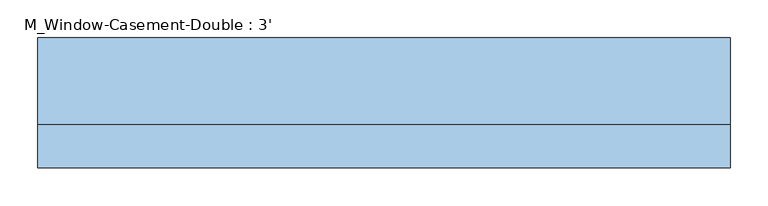
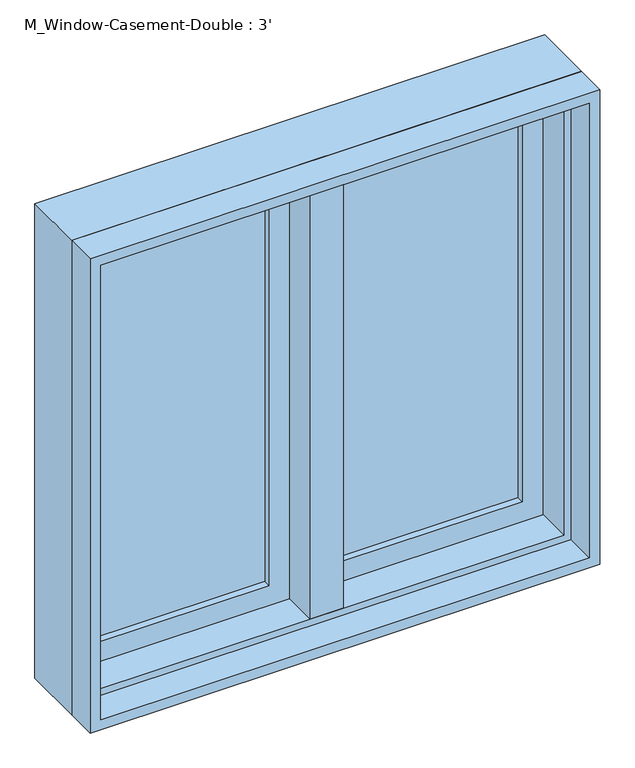
"""IFC4 building model written with IfcOpenShell, lengths in millimetres: window geometry, M_Window-Casement-Double : 3'."""

from ifc_helpers import new_model, si_unit, frame, origin, place, context, project, spatial, polyline, outline, extrude, faceted_brep, source, transform, mapped, element, save


def m_window_casement_double_3_e0bd8fa3(model_context):
    return source(origin(), model_context, "Body", "SolidModel", [
        faceted_brep([(425.45, 44.45, 1768.25), (425.45, -19.05, 1768.25), (-425.45, -19.05, 1768.25), (-425.45, 44.45, 1768.25), (444.5, 95.25, 1787.3), (444.5, 44.45, 1787.3), (-444.5, 44.45, 1787.3), (-444.5, 95.25, 1787.3), (457.2, -19.05, 1800.0), (457.2, 95.25, 1800.0), (-457.2, 95.25, 1800.0), (-457.2, -19.05, 1800.0), (-425.45, -19.05, 931.75), (-425.45, 44.45, 931.75), (-444.5, 44.45, 912.7), (-444.5, 95.25, 912.7), (-457.2, 95.25, 900.0), (-457.2, -19.05, 900.0), (425.45, -19.05, 931.75), (425.45, 44.45, 931.75), (444.5, 44.45, 912.7), (444.5, 95.25, 912.7), (457.2, 95.25, 900.0), (457.2, -19.05, 900.0)], [[[0, 1, 2, 3]], [[4, 5, 6, 7]], [[8, 9, 10, 11]], [[3, 2, 12, 13]], [[7, 6, 14, 15]], [[11, 10, 16, 17]], [[13, 12, 18, 19]], [[15, 14, 20, 21]], [[17, 16, 22, 23]], [[11, 17, 23, 8], [1, 18, 12, 2]], [[19, 18, 1, 0]], [[5, 20, 14, 6], [3, 13, 19, 0]], [[21, 20, 5, 4]], [[23, 22, 9, 8]], [[9, 22, 16, 10], [7, 15, 21, 4]]]),
        extrude(outline(polyline([(1800.0, -457.2), (900.0, -457.2), (900.0, 457.2), (1800.0, 457.2), (1800.0, -457.2)]), holes=[polyline([(1780.95, 438.15), (919.05, 438.15), (919.05, -438.15), (1780.95, -438.15), (1780.95, 438.15)])]), frame((0.0, -76.2, 0.0), z_axis=(0.0, 1.0, 0.0), x_axis=(0.0, 0.0, 1.0)), (0.0, 0.0, 1.0), 57.15),
        extrude(outline(polyline([(912.7, 444.5), (1787.3, 444.5), (1787.3, 9.525), (912.7, 9.525), (912.7, 444.5)]), holes=[polyline([(969.85, 66.675), (1730.15, 66.675), (1730.15, 387.35), (969.85, 387.35), (969.85, 66.675)])]), frame((0.0, 44.45, 0.0), z_axis=(0.0, 1.0, 0.0), x_axis=(0.0, 0.0, 1.0)), (0.0, 0.0, 1.0), 44.45),
        extrude(outline(polyline([(1787.3, -444.5), (912.7, -444.5), (912.7, -9.525), (1787.3, -9.525), (1787.3, -444.5)]), holes=[polyline([(1730.15, -66.675), (969.85, -66.675), (969.85, -387.35), (1730.15, -387.35), (1730.15, -66.675)])]), frame((0.0, 44.45, 0.0), z_axis=(0.0, 1.0, 0.0), x_axis=(0.0, 0.0, 1.0)), (0.0, 0.0, 1.0), 44.45),
        extrude(outline(polyline([(387.35, 76.2), (387.35, 69.85), (66.675, 69.85), (66.675, 76.2), (387.35, 76.2)])), frame((0.0, 0.0, 969.85), z_axis=(0.0, 0.0, 1.0), x_axis=(1.0, 0.0, 0.0)), (0.0, 0.0, 1.0), 760.3),
        extrude(outline(polyline([(66.675, 57.15), (66.675, 63.5), (387.35, 63.5), (387.35, 57.15), (66.675, 57.15)])), frame((0.0, 0.0, 969.85), z_axis=(0.0, 0.0, 1.0), x_axis=(1.0, 0.0, 0.0)), (0.0, 0.0, 1.0), 760.3),
        extrude(outline(polyline([(-66.675, 76.2), (-66.675, 69.85), (-387.35, 69.85), (-387.35, 76.2), (-66.675, 76.2)])), frame((0.0, 0.0, 969.85), z_axis=(0.0, 0.0, 1.0), x_axis=(1.0, 0.0, 0.0)), (0.0, 0.0, 1.0), 760.3),
        extrude(outline(polyline([(-387.35, 57.15), (-387.35, 63.5), (-66.675, 63.5), (-66.675, 57.15), (-387.35, 57.15)])), frame((0.0, 0.0, 969.85), z_axis=(0.0, 0.0, 1.0), x_axis=(1.0, 0.0, 0.0)), (0.0, 0.0, 1.0), 760.3),
        faceted_brep([(9.525, 95.25, 1787.3), (-9.525, 95.25, 1787.3), (-9.525, 44.45, 1787.3), (9.525, 44.45, 1787.3), (9.525, 95.25, 912.7), (9.525, 44.45, 912.7), (-9.525, 44.45, 912.7), (-9.525, 95.25, 912.7), (-9.525, 44.45, 931.75), (-9.525, 44.45, 1768.25), (-30.1625, 44.45, 931.75), (-30.1625, 44.45, 1768.25), (-30.1625, -19.05, 931.75), (-30.1625, -19.05, 1768.25), (30.1625, -19.05, 931.75), (30.1625, -19.05, 1768.25), (30.1625, 44.45, 931.75), (30.1625, 44.45, 1768.25), (9.525, 44.45, 931.75), (9.525, 44.45, 1768.25)], [[[0, 1, 2, 3]], [[4, 5, 6, 7]], [[1, 0, 4, 7]], [[2, 1, 7, 6, 8, 9]], [[9, 8, 10, 11]], [[11, 10, 12, 13]], [[13, 12, 14, 15]], [[15, 14, 16, 17]], [[17, 16, 18, 19]], [[0, 3, 19, 18, 5, 4]], [[18, 8, 6, 5]], [[9, 19, 3, 2]], [[8, 18, 16, 14, 12, 10]], [[19, 9, 11, 13, 15, 17]]]),
    ])


if __name__ == "__main__":
    model = new_model("IFC4")
    model_context = context("Model", 3, world=origin())
    ifc_project = project(units=[si_unit("LENGTHUNIT", "METRE", prefix="MILLI")], contexts=[model_context])
    site = spatial("IfcSite", under=ifc_project)
    building = spatial("IfcBuilding", under=site)
    placement = place(None, origin())
    m_window_casement_double_3_shape = m_window_casement_double_3_e0bd8fa3(model_context)
    element("IfcWindow", 1, ObjectType="M_Window-Casement-Double : 3'", at=placement, inside=building, context=model_context, shape_type="MappedRepresentation", body=[
        mapped(m_window_casement_double_3_shape, transform((0.0, 0.0, 0.0), x_axis=(1.0, 0.0, 0.0), y_axis=(0.0, 1.0, 0.0), z_axis=(0.0, 0.0, 1.0))),
    ])
    save(model, "model.ifc")

# Revit data of these elements
# Type "M_Window-Casement-Double : 3'"
#   Type Mark = "13"
#   Fire Rating = "0.5h"
#   Assembly Code = "B2020100"
#   Analytic Construction = "Double glazing - domestic"
#   Frame Extension [instance default] = 0' - 0 1/4"
#   Window Inset [instance default] = 0' - 0"
#   Wall Thickness [instance default] = 0' - 5.90551"
#   Interior Wall Closure [instance default] = 0' - 2.15551"
#   Half Width = 1' - 6"
#   Visual Light Transmittance = 0.81
#   Thermal Resistance (R) = 1.8146 (h·ft²·°F)/BTU
#   Solar Heat Gain Coefficient = 0.76
#   Rough Width = 3' - 0.59055"
#   Rough Height = 3' - 0.02362"
#   Height = 2' - 11.43307"
#   Heat Transfer Coefficient (U) = 0.5511 BTU/(h·ft²·°F)
#   Exterior Wall Closure [instance default] = 0' - 1.25197"
#   Extension Jamb [instance default] = 0' - 2.15551"
#   Default Sill Height = 2' - 11.43307"
#   Width = 3' - 0"
#   Muntin Visibility = yes
#   Interior Trim Visibility [instance default] = yes
#   Exterior Trim Visibility [instance default] = yes
#   Extension Jamb Visibility [instance default] = yes
#   Interior Trim Material = Wood - Stained
#   Muntin Pattern = M_Muntin Pattern_2x2 : M_Muntin Pattern_2x2
#   Interior Trim = M_Trim-Window-Interior-Flat : Picture Frame
#   Interior Frame Material = Wood - Stained
#   Glass Panel Material = Glass
#   Exterior Trim Material = Clad - White
#   Exterior Trim = M_Trim-Window-Exterior-Flat : with Sill
#   Exterior Frame Material = Clad - White
#   Wall Closure = (empty or 0)
# Element 1 (IfcWindow, "M_Window-Casement-Double : 3'")
#   Wall Thickness = 0' - 6"
#   Extension Jamb = 0' - 2 1/4"
#   Materials on its faces: "Wood - Stained", "Glass", "Clad - White"
# Materials
#   "Wood - Stained": class "Wood", colour RGB 227 170 128, transparency 0, Cost = 0
#   "Glass": class "Glass", colour RGB 218 227 224, transparency 0.85, Description = "Soda Lime Glass", Cost = 0
#   "Clad - White": class "Wood", colour RGB 242 242 238, transparency 0, Cost = 0
